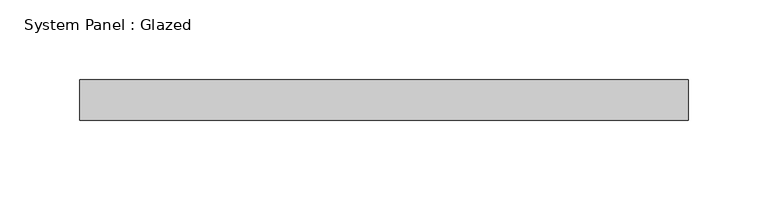
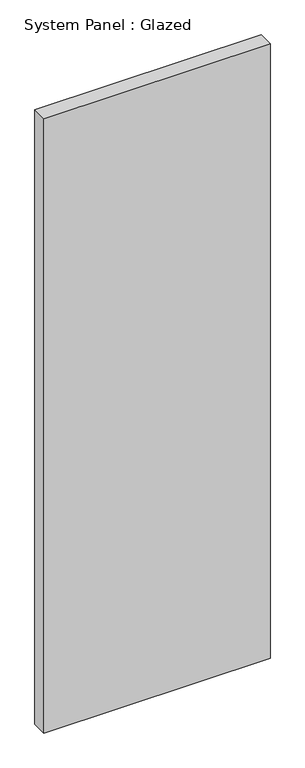
"""IFC4 building model written with IfcOpenShell, lengths in millimetres: plate geometry, System Panel : Glazed."""

from ifc_helpers import new_model, si_unit, origin, origin_with_axes, place, context, project, spatial, polyline, outline, extrude, source, transform, mapped, element, save


def system_panel_glazed_9262d402(model_context):
    return source(origin(), model_context, "Body", "SweptSolid", [
        extrude(outline(polyline([(190.3103194, 19.05), (-190.3103194, 19.05), (-190.3103194, 44.45), (190.3103194, 44.45), (190.3103194, 19.05)])), origin_with_axes(), (0.0, 0.0, 1.0), 1092.2),
    ])


if __name__ == "__main__":
    model = new_model("IFC4")
    model_context = context("Model", 3, world=origin())
    ifc_project = project(units=[si_unit("LENGTHUNIT", "METRE", prefix="MILLI")], contexts=[model_context])
    site = spatial("IfcSite", under=ifc_project)
    building = spatial("IfcBuilding", under=site)
    placement = place(None, origin())
    system_panel_glazed_shape = system_panel_glazed_9262d402(model_context)
    element("IfcPlate", 1, ObjectType="System Panel : Glazed", at=placement, inside=building, context=model_context, shape_type="MappedRepresentation", body=[
        mapped(system_panel_glazed_shape, transform((0.0, 0.0, 0.0), x_axis=(1.0, 0.0, 0.0), y_axis=(0.0, 1.0, 0.0), z_axis=(0.0, 0.0, 1.0))),
    ])
    save(model, "model.ifc")

# Revit data of these elements
# Type "System Panel : Glazed"
#   Construction Type Id = "GSP4R"
#   Analytic Construction = "1/8 in Pilkington single glazing"
#   Visual Light Transmittance = 0.9
#   Solar Heat Gain Coefficient = 0.86
#   Heat Transfer Coefficient (U) = 1.18115 BTU/(h·ft²·°F)
# Element 1 (IfcPlate, "System Panel : Glazed")
#   Materials on its faces: "Glass"
# Materials
#   "Glass": class "Glass", colour RGB 0 128 192, transparency 0.75, Description = "Soda Lime Glass", Cost = 0
